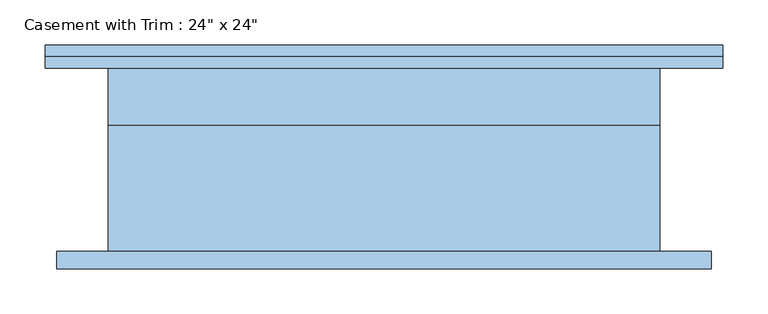
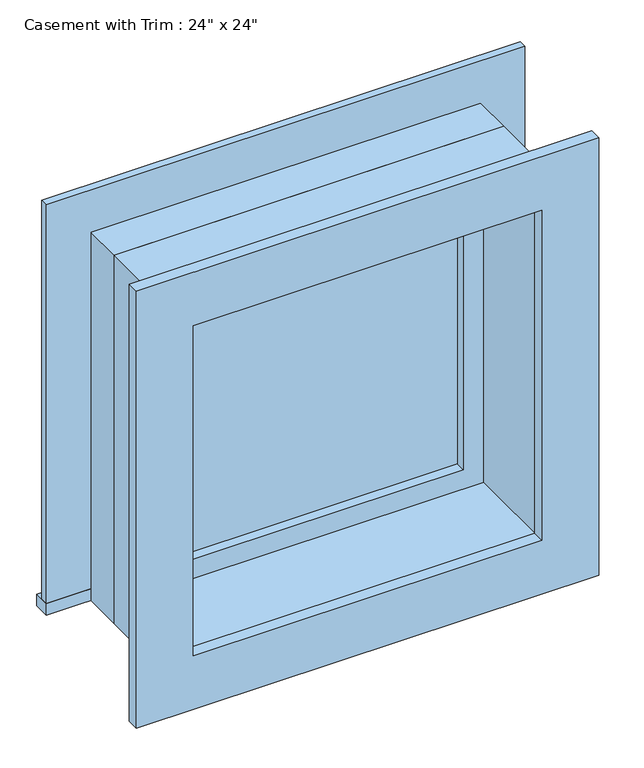
"""IFC4 building model written with IfcOpenShell, lengths in millimetres: window geometry."""

from ifc_helpers import new_model, si_unit, frame, origin, place, context, project, spatial, polyline, outline, extrude, source, transform, mapped, element, save


def window_3f0c7be2(model_context):
    return source(origin(), model_context, "Body", "SweptSolid", [
        extrude(outline(polyline([(-374.65, 127.0), (374.65, 127.0), (374.65, 101.6), (-374.65, 101.6), (-374.65, 127.0)])), frame((0.0, 0.0, 914.4), z_axis=(0.0, 0.0, 1.0), x_axis=(1.0, 0.0, 0.0)), (0.0, 0.0, 1.0), 19.05),
        extrude(outline(polyline([(1504.95, -285.75), (1504.95, 285.75), (933.45, 285.75), (933.45, 374.65), (1593.85, 374.65), (1593.85, -374.65), (933.45, -374.65), (933.45, -285.75), (1504.95, -285.75)])), frame((0.0, 101.6, 0.0), z_axis=(0.0, 1.0, 0.0), x_axis=(0.0, 0.0, 1.0)), (0.0, 0.0, 1.0), 12.7),
        extrude(outline(polyline([(1581.15, 361.95), (1581.15, -361.95), (857.25, -361.95), (857.25, 361.95), (1581.15, 361.95)]), holes=[polyline([(1492.25, 273.05), (946.15, 273.05), (946.15, -273.05), (1492.25, -273.05), (1492.25, 273.05)])]), frame((0.0, -120.65, 0.0), z_axis=(0.0, 1.0, 0.0), x_axis=(0.0, 0.0, 1.0)), (0.0, 0.0, 1.0), 19.05),
        extrude(outline(polyline([(241.3, 53.975), (-241.3, 53.975), (-241.3, 66.675), (241.3, 66.675), (241.3, 53.975)])), frame((0.0, 0.0, 977.9), z_axis=(0.0, 0.0, 1.0), x_axis=(1.0, 0.0, 0.0)), (0.0, 0.0, 1.0), 482.6),
        extrude(outline(polyline([(1504.95, -285.75), (933.45, -285.75), (933.45, 285.75), (1504.95, 285.75), (1504.95, -285.75)]), holes=[polyline([(1460.5, -241.3), (1460.5, 241.3), (977.9, 241.3), (977.9, -241.3), (1460.5, -241.3)])]), frame((0.0, 38.1, 0.0), z_axis=(0.0, 1.0, 0.0), x_axis=(0.0, 0.0, 1.0)), (0.0, 0.0, 1.0), 44.45),
        extrude(outline(polyline([(1524.0, -304.8), (914.4, -304.8), (914.4, 304.8), (1524.0, 304.8), (1524.0, -304.8)]), holes=[polyline([(1492.25, -273.05), (1492.25, 273.05), (946.15, 273.05), (946.15, -273.05), (1492.25, -273.05)])]), frame((0.0, -101.6, 0.0), z_axis=(0.0, 1.0, 0.0), x_axis=(0.0, 0.0, 1.0)), (0.0, 0.0, 1.0), 139.7),
        extrude(outline(polyline([(1524.0, 304.8), (1524.0, -304.8), (914.4, -304.8), (914.4, 304.8), (1524.0, 304.8)]), holes=[polyline([(1504.95, 285.75), (933.45, 285.75), (933.45, -285.75), (1504.95, -285.75), (1504.95, 285.75)])]), frame((0.0, 38.1, 0.0), z_axis=(0.0, 1.0, 0.0), x_axis=(0.0, 0.0, 1.0)), (0.0, 0.0, 1.0), 63.5),
    ])


if __name__ == "__main__":
    model = new_model("IFC4")
    model_context = context("Model", 3, world=origin())
    ifc_project = project(units=[si_unit("LENGTHUNIT", "METRE", prefix="MILLI")], contexts=[model_context])
    site = spatial("IfcSite", under=ifc_project)
    building = spatial("IfcBuilding", under=site)
    placement = place(None, origin())
    window_shape = window_3f0c7be2(model_context)
    element("IfcWindow", 1, ObjectType="Casement with Trim : 24\" x 24\"", at=placement, inside=building, context=model_context, shape_type="MappedRepresentation", body=[
        mapped(window_shape, transform((0.0, 0.0, 0.0), x_axis=(1.0, 0.0, 0.0), y_axis=(0.0, 1.0, 0.0), z_axis=(0.0, 0.0, 1.0))),
    ])
    save(model, "model.ifc")

# Revit data of these elements
# Type "Casement with Trim : 24\" x 24\""
#   Type Mark = "28"
#   Construction Type Id = "GSP4R"
#   Assembly Code = "B2020100"
#   Analytic Construction = "1/8 in Pilkington single glazing"
#   Visual Light Transmittance = 0.9
#   Solar Heat Gain Coefficient = 0.78
#   Heat Transfer Coefficient (U) = 0.6496 BTU/(h·ft²·°F)
#   Height = 2' - 0"
#   Default Sill Height = 3' - 0"
#   Trim Projection - Ext. = 0' - 0 1/2"
#   Trim Projection - Int. = 0' - 0 3/4"
#   Trim Width - Exterior = 0' - 3 1/2"
#   Trim Width - Interior = 0' - 3 1/2"
#   Width = 2' - 0"
#   Window Inset = 0' - 0 3/4"
#   Define Thermal Properties by = 1
#   Glass Pane Material = Glass
#   Sash Material = Sash
#   Trim Exterior Material = Trim
#   Trim Interior Material = Trim
#   Wall Closure = (empty or 0)
# Element 1 (IfcWindow, "Casement with Trim : 24\" x 24\"")
#   Materials on its faces: "Sash", "Trim", "Glass"
# Materials
#   "Glass": class "Glass", colour RGB 0 128 192, transparency 0.75, Description = "Soda Lime Glass", Cost = 0
#   "Sash": class "Wood", colour RGB 224 178 126, transparency 0
#   "Trim": class "Wood", colour RGB 224 178 126, transparency 0
